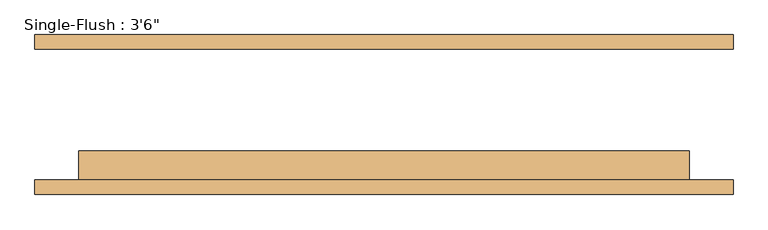
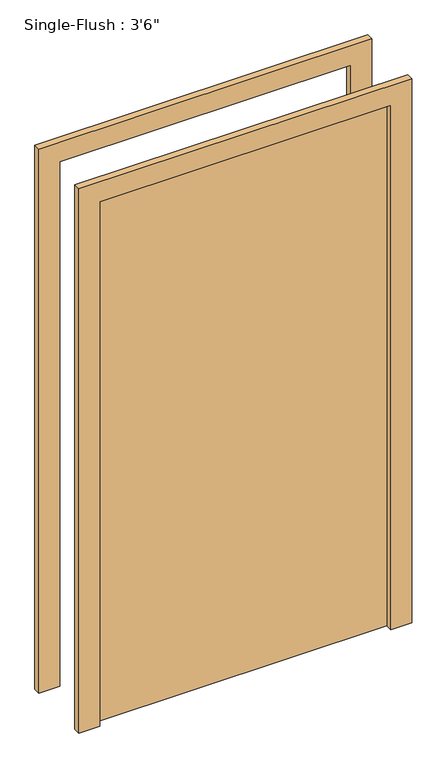
"""IFC4 building model written with IfcOpenShell, lengths in millimetres: door geometry."""

from ifc_helpers import new_model, si_unit, frame, origin, origin_with_axes, place, context, project, spatial, polyline, outline, extrude, source, transform, mapped, element, save


def door_f6232a3f(model_context):
    return source(origin(), model_context, "Body", "SweptSolid", [
        extrude(outline(polyline([(2108.2, -609.6), (0.0, -609.6), (0.0, -533.4), (2032.0, -533.4), (2032.0, 533.4), (0.0, 533.4), (0.0, 609.6), (2108.2, 609.6), (2108.2, -609.6)])), frame((0.0, -139.7, 0.0), z_axis=(0.0, 1.0, 0.0), x_axis=(0.0, 0.0, 1.0)), (0.0, 0.0, 1.0), 25.4),
        extrude(outline(polyline([(2108.2, 609.6), (2108.2, -609.6), (0.0, -609.6), (0.0, -533.4), (2032.0, -533.4), (2032.0, 533.4), (0.0, 533.4), (0.0, 609.6), (2108.2, 609.6)])), frame((0.0, 114.3, 0.0), z_axis=(0.0, 1.0, 0.0), x_axis=(0.0, 0.0, 1.0)), (0.0, 0.0, 1.0), 25.4),
        extrude(outline(polyline([(533.4, -63.5), (533.4, -114.3), (-533.4, -114.3), (-533.4, -63.5), (533.4, -63.5)])), origin_with_axes(), (0.0, 0.0, 1.0), 2032.0),
    ])


if __name__ == "__main__":
    model = new_model("IFC4")
    model_context = context("Model", 3, world=origin())
    ifc_project = project(units=[si_unit("LENGTHUNIT", "METRE", prefix="MILLI")], contexts=[model_context])
    site = spatial("IfcSite", under=ifc_project)
    building = spatial("IfcBuilding", under=site)
    placement = place(None, origin())
    door_shape = door_f6232a3f(model_context)
    element("IfcDoor", 1, ObjectType="Single-Flush : 3'6\"", at=placement, inside=building, context=model_context, shape_type="MappedRepresentation", body=[
        mapped(door_shape, transform((0.0, 0.0, 0.0), x_axis=(1.0, 0.0, 0.0), y_axis=(0.0, 1.0, 0.0), z_axis=(0.0, 0.0, 1.0))),
    ])
    save(model, "model.ifc")

# Revit data of these elements
# Type "Single-Flush : 3'6\""
#   Type Mark = "11"
#   Construction Type Id = "MDOOR"
#   Assembly Code = "C1020"
#   Analytic Construction = "Metal"
#   Thickness = 0' - 2"
#   Heat Transfer Coefficient (U) = 0.651978 BTU/(h·ft²·°F)
#   Height = 6' - 8"
#   Trim Projection Ext = 0' - 1"
#   Trim Projection Int = 0' - 1"
#   Trim Width = 0' - 3"
#   Width = 3' - 6"
#   Define Thermal Properties by = 1
#   Door Material = Door - Panel
#   Frame Material = Door - Frame
#   Visual Light Transmittance = 0
#   Solar Heat Gain Coefficient = 0
#   Function = (empty or 0)
#   Wall Closure = (empty or 0)
# Element 1 (IfcDoor, "Single-Flush : 3'6\"")
#   Materials on its faces: "Door - Frame", "Door - Panel"
# Materials
#   "Door - Panel": class "Wood", colour RGB 210 159 95, transparency 0, Cost = 0
#   "Door - Frame": colour RGB 118 70 51, transparency 0, Cost = 0
